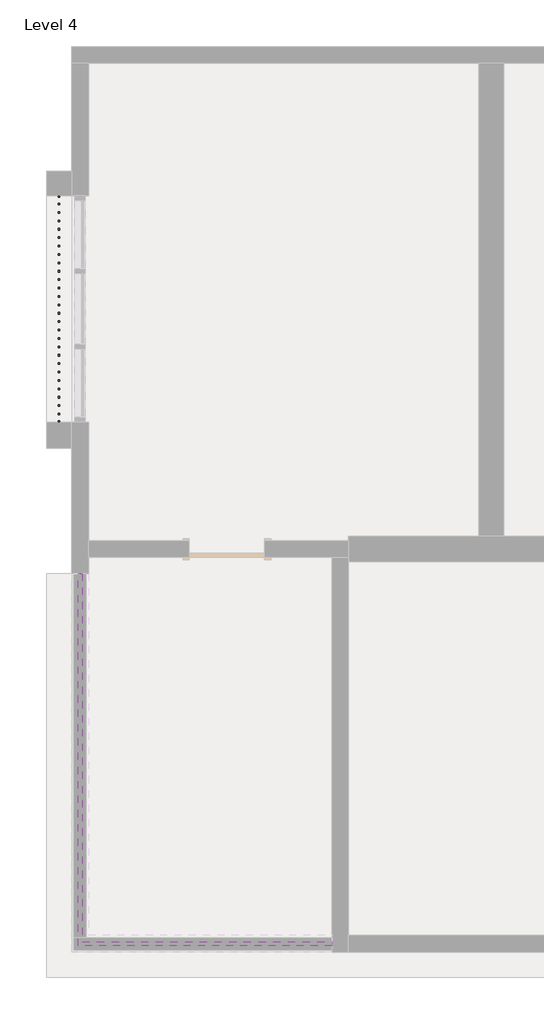
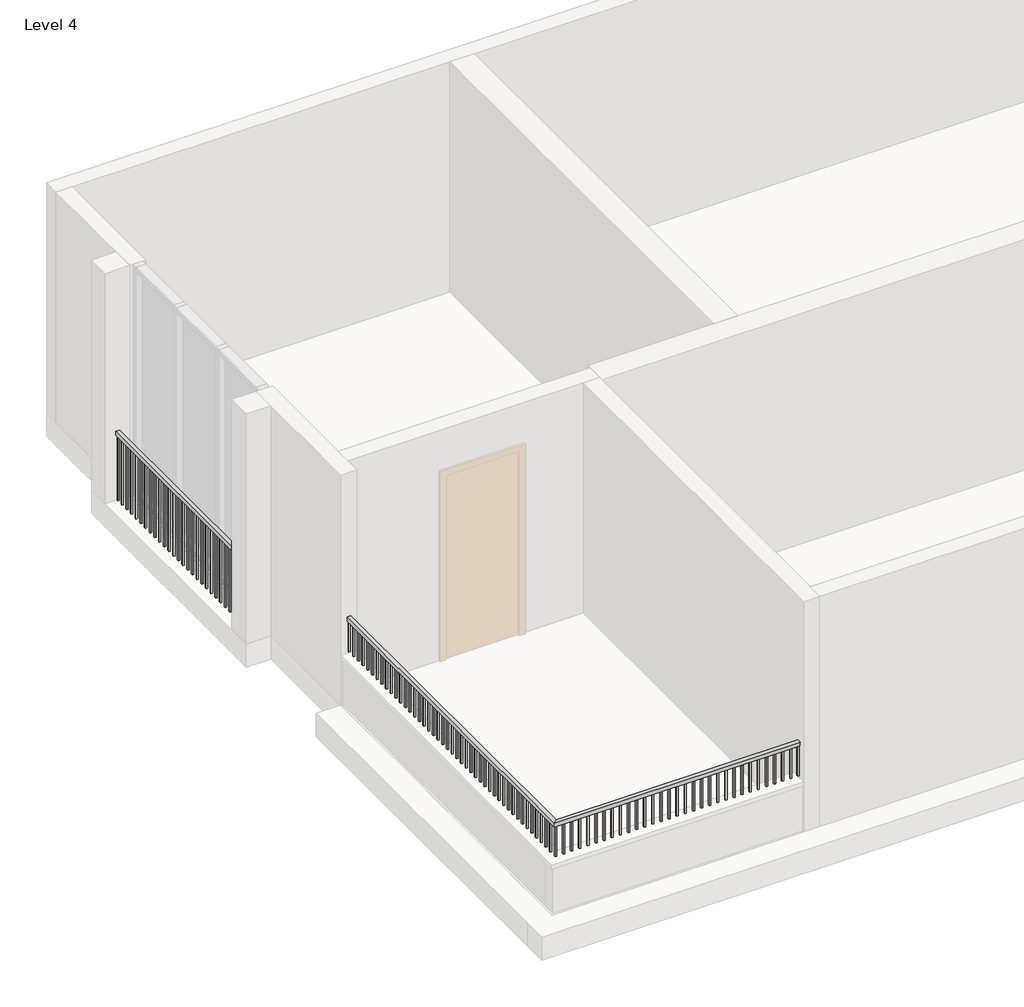
# One storey, part 2 of 2: 2 railings.
"""IFC4 building model written with IfcOpenShell, lengths in millimetres."""

from ifc_helpers import new_model, si_unit, frame, origin, place, context, project, spatial, polyline, outline, extrude, faceted_brep, element, save

model = new_model("IFC4")

# Units and contexts
model_context = context("Model", 3, world=origin())
ifc_project = project(units=[si_unit("LENGTHUNIT", "METRE", prefix="MILLI")], contexts=[model_context])

# Site, building, storey
site = spatial("IfcSite", under=ifc_project)
building = spatial("IfcBuilding", under=site)
storey = spatial("IfcBuildingStorey", under=building, Name="Level 4", Elevation=9144.0)

# Railings
placement = place(None, origin())
element("IfcRailing", 1, ObjectType="Handrail - Rectangular", at=placement, inside=storey, context=model_context, shape_type="SolidModel", body=[
    faceted_brep([(-15179.2169582, -9411.0617616, 11201.4), (-15179.2169582, -9411.0617616, 11150.6), (-15179.2169582, -9360.2617616, 11150.6), (-15179.2169582, -9360.2617616, 11201.4), (-18252.6169582, -9411.0617616, 11201.4), (-18252.6169582, -9411.0617616, 11150.6), (-18201.8169582, -9360.2617616, 11150.6), (-18201.8169582, -9360.2617616, 11201.4), (-18252.6169582, -4908.9117616, 11201.4), (-18201.8169582, -4908.9117616, 11201.4), (-18201.8169582, -4908.9117616, 11150.6), (-18252.6169582, -4908.9117616, 11150.6)], [[[0, 1, 2, 3]], [[1, 0, 4, 5]], [[2, 1, 5, 6]], [[3, 2, 6, 7]], [[0, 3, 7, 4]], [[8, 9, 10, 11]], [[5, 4, 8, 11]], [[6, 5, 11, 10]], [[7, 6, 10, 9]], [[4, 7, 9, 8]]]),
    extrude(outline(polyline([(-18217.6919582, -4924.7867616), (-18236.7419582, -4924.7867616), (-18236.7419582, -4905.7367616), (-18217.6919582, -4905.7367616), (-18217.6919582, -4924.7867616)])), frame((0.0, 0.0, 10744.2), z_axis=(0.0, 0.0, 1.0), x_axis=(1.0, 0.0, 0.0)), (0.0, 0.0, 1.0), 406.4),
    extrude(outline(polyline([(-18217.6919582, -5026.3867616), (-18236.7419582, -5026.3867616), (-18236.7419582, -5007.3367616), (-18217.6919582, -5007.3367616), (-18217.6919582, -5026.3867616)])), frame((0.0, 0.0, 10744.2), z_axis=(0.0, 0.0, 1.0), x_axis=(1.0, 0.0, 0.0)), (0.0, 0.0, 1.0), 406.4),
    extrude(outline(polyline([(-18217.6919582, -5127.9867616), (-18236.7419582, -5127.9867616), (-18236.7419582, -5108.9367616), (-18217.6919582, -5108.9367616), (-18217.6919582, -5127.9867616)])), frame((0.0, 0.0, 10744.2), z_axis=(0.0, 0.0, 1.0), x_axis=(1.0, 0.0, 0.0)), (0.0, 0.0, 1.0), 406.4),
    extrude(outline(polyline([(-18217.6919582, -5229.5867616), (-18236.7419582, -5229.5867616), (-18236.7419582, -5210.5367616), (-18217.6919582, -5210.5367616), (-18217.6919582, -5229.5867616)])), frame((0.0, 0.0, 10744.2), z_axis=(0.0, 0.0, 1.0), x_axis=(1.0, 0.0, 0.0)), (0.0, 0.0, 1.0), 406.4),
    extrude(outline(polyline([(-18217.6919582, -5331.1867616), (-18236.7419582, -5331.1867616), (-18236.7419582, -5312.1367616), (-18217.6919582, -5312.1367616), (-18217.6919582, -5331.1867616)])), frame((0.0, 0.0, 10744.2), z_axis=(0.0, 0.0, 1.0), x_axis=(1.0, 0.0, 0.0)), (0.0, 0.0, 1.0), 406.4),
    extrude(outline(polyline([(-18217.6919582, -5432.7867616), (-18236.7419582, -5432.7867616), (-18236.7419582, -5413.7367616), (-18217.6919582, -5413.7367616), (-18217.6919582, -5432.7867616)])), frame((0.0, 0.0, 10744.2), z_axis=(0.0, 0.0, 1.0), x_axis=(1.0, 0.0, 0.0)), (0.0, 0.0, 1.0), 406.4),
    extrude(outline(polyline([(-18217.6919582, -5534.3867616), (-18236.7419582, -5534.3867616), (-18236.7419582, -5515.3367616), (-18217.6919582, -5515.3367616), (-18217.6919582, -5534.3867616)])), frame((0.0, 0.0, 10744.2), z_axis=(0.0, 0.0, 1.0), x_axis=(1.0, 0.0, 0.0)), (0.0, 0.0, 1.0), 406.4),
    extrude(outline(polyline([(-18217.6919582, -5635.9867616), (-18236.7419582, -5635.9867616), (-18236.7419582, -5616.9367616), (-18217.6919582, -5616.9367616), (-18217.6919582, -5635.9867616)])), frame((0.0, 0.0, 10744.2), z_axis=(0.0, 0.0, 1.0), x_axis=(1.0, 0.0, 0.0)), (0.0, 0.0, 1.0), 406.4),
    extrude(outline(polyline([(-18217.6919582, -5737.5867616), (-18236.7419582, -5737.5867616), (-18236.7419582, -5718.5367616), (-18217.6919582, -5718.5367616), (-18217.6919582, -5737.5867616)])), frame((0.0, 0.0, 10744.2), z_axis=(0.0, 0.0, 1.0), x_axis=(1.0, 0.0, 0.0)), (0.0, 0.0, 1.0), 406.4),
    extrude(outline(polyline([(-18217.6919582, -5839.1867616), (-18236.7419582, -5839.1867616), (-18236.7419582, -5820.1367616), (-18217.6919582, -5820.1367616), (-18217.6919582, -5839.1867616)])), frame((0.0, 0.0, 10744.2), z_axis=(0.0, 0.0, 1.0), x_axis=(1.0, 0.0, 0.0)), (0.0, 0.0, 1.0), 406.4),
    extrude(outline(polyline([(-18217.6919582, -5940.7867616), (-18236.7419582, -5940.7867616), (-18236.7419582, -5921.7367616), (-18217.6919582, -5921.7367616), (-18217.6919582, -5940.7867616)])), frame((0.0, 0.0, 10744.2), z_axis=(0.0, 0.0, 1.0), x_axis=(1.0, 0.0, 0.0)), (0.0, 0.0, 1.0), 406.4),
    extrude(outline(polyline([(-18217.6919582, -6042.3867616), (-18236.7419582, -6042.3867616), (-18236.7419582, -6023.3367616), (-18217.6919582, -6023.3367616), (-18217.6919582, -6042.3867616)])), frame((0.0, 0.0, 10744.2), z_axis=(0.0, 0.0, 1.0), x_axis=(1.0, 0.0, 0.0)), (0.0, 0.0, 1.0), 406.4),
    extrude(outline(polyline([(-18217.6919582, -6143.9867616), (-18236.7419582, -6143.9867616), (-18236.7419582, -6124.9367616), (-18217.6919582, -6124.9367616), (-18217.6919582, -6143.9867616)])), frame((0.0, 0.0, 10744.2), z_axis=(0.0, 0.0, 1.0), x_axis=(1.0, 0.0, 0.0)), (0.0, 0.0, 1.0), 406.4),
    extrude(outline(polyline([(-18217.6919582, -6245.5867616), (-18236.7419582, -6245.5867616), (-18236.7419582, -6226.5367616), (-18217.6919582, -6226.5367616), (-18217.6919582, -6245.5867616)])), frame((0.0, 0.0, 10744.2), z_axis=(0.0, 0.0, 1.0), x_axis=(1.0, 0.0, 0.0)), (0.0, 0.0, 1.0), 406.4),
    extrude(outline(polyline([(-18217.6919582, -6347.1867616), (-18236.7419582, -6347.1867616), (-18236.7419582, -6328.1367616), (-18217.6919582, -6328.1367616), (-18217.6919582, -6347.1867616)])), frame((0.0, 0.0, 10744.2), z_axis=(0.0, 0.0, 1.0), x_axis=(1.0, 0.0, 0.0)), (0.0, 0.0, 1.0), 406.4),
    extrude(outline(polyline([(-18217.6919582, -6448.7867616), (-18236.7419582, -6448.7867616), (-18236.7419582, -6429.7367616), (-18217.6919582, -6429.7367616), (-18217.6919582, -6448.7867616)])), frame((0.0, 0.0, 10744.2), z_axis=(0.0, 0.0, 1.0), x_axis=(1.0, 0.0, 0.0)), (0.0, 0.0, 1.0), 406.4),
    extrude(outline(polyline([(-18217.6919582, -6550.3867616), (-18236.7419582, -6550.3867616), (-18236.7419582, -6531.3367616), (-18217.6919582, -6531.3367616), (-18217.6919582, -6550.3867616)])), frame((0.0, 0.0, 10744.2), z_axis=(0.0, 0.0, 1.0), x_axis=(1.0, 0.0, 0.0)), (0.0, 0.0, 1.0), 406.4),
    extrude(outline(polyline([(-18217.6919582, -6651.9867616), (-18236.7419582, -6651.9867616), (-18236.7419582, -6632.9367616), (-18217.6919582, -6632.9367616), (-18217.6919582, -6651.9867616)])), frame((0.0, 0.0, 10744.2), z_axis=(0.0, 0.0, 1.0), x_axis=(1.0, 0.0, 0.0)), (0.0, 0.0, 1.0), 406.4),
    extrude(outline(polyline([(-18217.6919582, -6753.5867616), (-18236.7419582, -6753.5867616), (-18236.7419582, -6734.5367616), (-18217.6919582, -6734.5367616), (-18217.6919582, -6753.5867616)])), frame((0.0, 0.0, 10744.2), z_axis=(0.0, 0.0, 1.0), x_axis=(1.0, 0.0, 0.0)), (0.0, 0.0, 1.0), 406.4),
    extrude(outline(polyline([(-18217.6919582, -6855.1867616), (-18236.7419582, -6855.1867616), (-18236.7419582, -6836.1367616), (-18217.6919582, -6836.1367616), (-18217.6919582, -6855.1867616)])), frame((0.0, 0.0, 10744.2), z_axis=(0.0, 0.0, 1.0), x_axis=(1.0, 0.0, 0.0)), (0.0, 0.0, 1.0), 406.4),
    extrude(outline(polyline([(-18217.6919582, -6956.7867616), (-18236.7419582, -6956.7867616), (-18236.7419582, -6937.7367616), (-18217.6919582, -6937.7367616), (-18217.6919582, -6956.7867616)])), frame((0.0, 0.0, 10744.2), z_axis=(0.0, 0.0, 1.0), x_axis=(1.0, 0.0, 0.0)), (0.0, 0.0, 1.0), 406.4),
    extrude(outline(polyline([(-18217.6919582, -7058.3867616), (-18236.7419582, -7058.3867616), (-18236.7419582, -7039.3367616), (-18217.6919582, -7039.3367616), (-18217.6919582, -7058.3867616)])), frame((0.0, 0.0, 10744.2), z_axis=(0.0, 0.0, 1.0), x_axis=(1.0, 0.0, 0.0)), (0.0, 0.0, 1.0), 406.4),
    extrude(outline(polyline([(-18217.6919582, -7159.9867616), (-18236.7419582, -7159.9867616), (-18236.7419582, -7140.9367616), (-18217.6919582, -7140.9367616), (-18217.6919582, -7159.9867616)])), frame((0.0, 0.0, 10744.2), z_axis=(0.0, 0.0, 1.0), x_axis=(1.0, 0.0, 0.0)), (0.0, 0.0, 1.0), 406.4),
    extrude(outline(polyline([(-18217.6919582, -7261.5867616), (-18236.7419582, -7261.5867616), (-18236.7419582, -7242.5367616), (-18217.6919582, -7242.5367616), (-18217.6919582, -7261.5867616)])), frame((0.0, 0.0, 10744.2), z_axis=(0.0, 0.0, 1.0), x_axis=(1.0, 0.0, 0.0)), (0.0, 0.0, 1.0), 406.4),
    extrude(outline(polyline([(-18217.6919582, -7363.1867616), (-18236.7419582, -7363.1867616), (-18236.7419582, -7344.1367616), (-18217.6919582, -7344.1367616), (-18217.6919582, -7363.1867616)])), frame((0.0, 0.0, 10744.2), z_axis=(0.0, 0.0, 1.0), x_axis=(1.0, 0.0, 0.0)), (0.0, 0.0, 1.0), 406.4),
    extrude(outline(polyline([(-18217.6919582, -7464.7867616), (-18236.7419582, -7464.7867616), (-18236.7419582, -7445.7367616), (-18217.6919582, -7445.7367616), (-18217.6919582, -7464.7867616)])), frame((0.0, 0.0, 10744.2), z_axis=(0.0, 0.0, 1.0), x_axis=(1.0, 0.0, 0.0)), (0.0, 0.0, 1.0), 406.4),
    extrude(outline(polyline([(-18217.6919582, -7566.3867616), (-18236.7419582, -7566.3867616), (-18236.7419582, -7547.3367616), (-18217.6919582, -7547.3367616), (-18217.6919582, -7566.3867616)])), frame((0.0, 0.0, 10744.2), z_axis=(0.0, 0.0, 1.0), x_axis=(1.0, 0.0, 0.0)), (0.0, 0.0, 1.0), 406.4),
    extrude(outline(polyline([(-18217.6919582, -7667.9867616), (-18236.7419582, -7667.9867616), (-18236.7419582, -7648.9367616), (-18217.6919582, -7648.9367616), (-18217.6919582, -7667.9867616)])), frame((0.0, 0.0, 10744.2), z_axis=(0.0, 0.0, 1.0), x_axis=(1.0, 0.0, 0.0)), (0.0, 0.0, 1.0), 406.4),
    extrude(outline(polyline([(-18217.6919582, -7769.5867616), (-18236.7419582, -7769.5867616), (-18236.7419582, -7750.5367616), (-18217.6919582, -7750.5367616), (-18217.6919582, -7769.5867616)])), frame((0.0, 0.0, 10744.2), z_axis=(0.0, 0.0, 1.0), x_axis=(1.0, 0.0, 0.0)), (0.0, 0.0, 1.0), 406.4),
    extrude(outline(polyline([(-18217.6919582, -7871.1867616), (-18236.7419582, -7871.1867616), (-18236.7419582, -7852.1367616), (-18217.6919582, -7852.1367616), (-18217.6919582, -7871.1867616)])), frame((0.0, 0.0, 10744.2), z_axis=(0.0, 0.0, 1.0), x_axis=(1.0, 0.0, 0.0)), (0.0, 0.0, 1.0), 406.4),
    extrude(outline(polyline([(-18217.6919582, -7972.7867616), (-18236.7419582, -7972.7867616), (-18236.7419582, -7953.7367616), (-18217.6919582, -7953.7367616), (-18217.6919582, -7972.7867616)])), frame((0.0, 0.0, 10744.2), z_axis=(0.0, 0.0, 1.0), x_axis=(1.0, 0.0, 0.0)), (0.0, 0.0, 1.0), 406.4),
    extrude(outline(polyline([(-18217.6919582, -8074.3867616), (-18236.7419582, -8074.3867616), (-18236.7419582, -8055.3367616), (-18217.6919582, -8055.3367616), (-18217.6919582, -8074.3867616)])), frame((0.0, 0.0, 10744.2), z_axis=(0.0, 0.0, 1.0), x_axis=(1.0, 0.0, 0.0)), (0.0, 0.0, 1.0), 406.4),
    extrude(outline(polyline([(-18217.6919582, -8175.9867616), (-18236.7419582, -8175.9867616), (-18236.7419582, -8156.9367616), (-18217.6919582, -8156.9367616), (-18217.6919582, -8175.9867616)])), frame((0.0, 0.0, 10744.2), z_axis=(0.0, 0.0, 1.0), x_axis=(1.0, 0.0, 0.0)), (0.0, 0.0, 1.0), 406.4),
    extrude(outline(polyline([(-18217.6919582, -8277.5867616), (-18236.7419582, -8277.5867616), (-18236.7419582, -8258.5367616), (-18217.6919582, -8258.5367616), (-18217.6919582, -8277.5867616)])), frame((0.0, 0.0, 10744.2), z_axis=(0.0, 0.0, 1.0), x_axis=(1.0, 0.0, 0.0)), (0.0, 0.0, 1.0), 406.4),
    extrude(outline(polyline([(-18217.6919582, -8379.1867616), (-18236.7419582, -8379.1867616), (-18236.7419582, -8360.1367616), (-18217.6919582, -8360.1367616), (-18217.6919582, -8379.1867616)])), frame((0.0, 0.0, 10744.2), z_axis=(0.0, 0.0, 1.0), x_axis=(1.0, 0.0, 0.0)), (0.0, 0.0, 1.0), 406.4),
    extrude(outline(polyline([(-18217.6919582, -8480.7867616), (-18236.7419582, -8480.7867616), (-18236.7419582, -8461.7367616), (-18217.6919582, -8461.7367616), (-18217.6919582, -8480.7867616)])), frame((0.0, 0.0, 10744.2), z_axis=(0.0, 0.0, 1.0), x_axis=(1.0, 0.0, 0.0)), (0.0, 0.0, 1.0), 406.4),
    extrude(outline(polyline([(-18217.6919582, -8582.3867616), (-18236.7419582, -8582.3867616), (-18236.7419582, -8563.3367616), (-18217.6919582, -8563.3367616), (-18217.6919582, -8582.3867616)])), frame((0.0, 0.0, 10744.2), z_axis=(0.0, 0.0, 1.0), x_axis=(1.0, 0.0, 0.0)), (0.0, 0.0, 1.0), 406.4),
    extrude(outline(polyline([(-18217.6919582, -8683.9867616), (-18236.7419582, -8683.9867616), (-18236.7419582, -8664.9367616), (-18217.6919582, -8664.9367616), (-18217.6919582, -8683.9867616)])), frame((0.0, 0.0, 10744.2), z_axis=(0.0, 0.0, 1.0), x_axis=(1.0, 0.0, 0.0)), (0.0, 0.0, 1.0), 406.4),
    extrude(outline(polyline([(-18217.6919582, -8785.5867616), (-18236.7419582, -8785.5867616), (-18236.7419582, -8766.5367616), (-18217.6919582, -8766.5367616), (-18217.6919582, -8785.5867616)])), frame((0.0, 0.0, 10744.2), z_axis=(0.0, 0.0, 1.0), x_axis=(1.0, 0.0, 0.0)), (0.0, 0.0, 1.0), 406.4),
    extrude(outline(polyline([(-18217.6919582, -8887.1867616), (-18236.7419582, -8887.1867616), (-18236.7419582, -8868.1367616), (-18217.6919582, -8868.1367616), (-18217.6919582, -8887.1867616)])), frame((0.0, 0.0, 10744.2), z_axis=(0.0, 0.0, 1.0), x_axis=(1.0, 0.0, 0.0)), (0.0, 0.0, 1.0), 406.4),
    extrude(outline(polyline([(-18217.6919582, -8988.7867616), (-18236.7419582, -8988.7867616), (-18236.7419582, -8969.7367616), (-18217.6919582, -8969.7367616), (-18217.6919582, -8988.7867616)])), frame((0.0, 0.0, 10744.2), z_axis=(0.0, 0.0, 1.0), x_axis=(1.0, 0.0, 0.0)), (0.0, 0.0, 1.0), 406.4),
    extrude(outline(polyline([(-18217.6919582, -9090.3867616), (-18236.7419582, -9090.3867616), (-18236.7419582, -9071.3367616), (-18217.6919582, -9071.3367616), (-18217.6919582, -9090.3867616)])), frame((0.0, 0.0, 10744.2), z_axis=(0.0, 0.0, 1.0), x_axis=(1.0, 0.0, 0.0)), (0.0, 0.0, 1.0), 406.4),
    extrude(outline(polyline([(-18217.6919582, -9191.9867616), (-18236.7419582, -9191.9867616), (-18236.7419582, -9172.9367616), (-18217.6919582, -9172.9367616), (-18217.6919582, -9191.9867616)])), frame((0.0, 0.0, 10744.2), z_axis=(0.0, 0.0, 1.0), x_axis=(1.0, 0.0, 0.0)), (0.0, 0.0, 1.0), 406.4),
    extrude(outline(polyline([(-18217.6919582, -9293.5867616), (-18236.7419582, -9293.5867616), (-18236.7419582, -9274.5367616), (-18217.6919582, -9274.5367616), (-18217.6919582, -9293.5867616)])), frame((0.0, 0.0, 10744.2), z_axis=(0.0, 0.0, 1.0), x_axis=(1.0, 0.0, 0.0)), (0.0, 0.0, 1.0), 406.4),
    extrude(outline(polyline([(-18116.0919582, -9376.1367616), (-18116.0919582, -9395.1867616), (-18135.1419582, -9395.1867616), (-18135.1419582, -9376.1367616), (-18116.0919582, -9376.1367616)])), frame((0.0, 0.0, 10744.2), z_axis=(0.0, 0.0, 1.0), x_axis=(1.0, 0.0, 0.0)), (0.0, 0.0, 1.0), 406.4),
    extrude(outline(polyline([(-18014.4919582, -9376.1367616), (-18014.4919582, -9395.1867616), (-18033.5419582, -9395.1867616), (-18033.5419582, -9376.1367616), (-18014.4919582, -9376.1367616)])), frame((0.0, 0.0, 10744.2), z_axis=(0.0, 0.0, 1.0), x_axis=(1.0, 0.0, 0.0)), (0.0, 0.0, 1.0), 406.4),
    extrude(outline(polyline([(-17912.8919582, -9376.1367616), (-17912.8919582, -9395.1867616), (-17931.9419582, -9395.1867616), (-17931.9419582, -9376.1367616), (-17912.8919582, -9376.1367616)])), frame((0.0, 0.0, 10744.2), z_axis=(0.0, 0.0, 1.0), x_axis=(1.0, 0.0, 0.0)), (0.0, 0.0, 1.0), 406.4),
    extrude(outline(polyline([(-17811.2919582, -9376.1367616), (-17811.2919582, -9395.1867616), (-17830.3419582, -9395.1867616), (-17830.3419582, -9376.1367616), (-17811.2919582, -9376.1367616)])), frame((0.0, 0.0, 10744.2), z_axis=(0.0, 0.0, 1.0), x_axis=(1.0, 0.0, 0.0)), (0.0, 0.0, 1.0), 406.4),
    extrude(outline(polyline([(-17709.6919582, -9376.1367616), (-17709.6919582, -9395.1867616), (-17728.7419582, -9395.1867616), (-17728.7419582, -9376.1367616), (-17709.6919582, -9376.1367616)])), frame((0.0, 0.0, 10744.2), z_axis=(0.0, 0.0, 1.0), x_axis=(1.0, 0.0, 0.0)), (0.0, 0.0, 1.0), 406.4),
    extrude(outline(polyline([(-17608.0919582, -9376.1367616), (-17608.0919582, -9395.1867616), (-17627.1419582, -9395.1867616), (-17627.1419582, -9376.1367616), (-17608.0919582, -9376.1367616)])), frame((0.0, 0.0, 10744.2), z_axis=(0.0, 0.0, 1.0), x_axis=(1.0, 0.0, 0.0)), (0.0, 0.0, 1.0), 406.4),
    extrude(outline(polyline([(-17506.4919582, -9376.1367616), (-17506.4919582, -9395.1867616), (-17525.5419582, -9395.1867616), (-17525.5419582, -9376.1367616), (-17506.4919582, -9376.1367616)])), frame((0.0, 0.0, 10744.2), z_axis=(0.0, 0.0, 1.0), x_axis=(1.0, 0.0, 0.0)), (0.0, 0.0, 1.0), 406.4),
    extrude(outline(polyline([(-17404.8919582, -9376.1367616), (-17404.8919582, -9395.1867616), (-17423.9419582, -9395.1867616), (-17423.9419582, -9376.1367616), (-17404.8919582, -9376.1367616)])), frame((0.0, 0.0, 10744.2), z_axis=(0.0, 0.0, 1.0), x_axis=(1.0, 0.0, 0.0)), (0.0, 0.0, 1.0), 406.4),
    extrude(outline(polyline([(-17303.2919582, -9376.1367616), (-17303.2919582, -9395.1867616), (-17322.3419582, -9395.1867616), (-17322.3419582, -9376.1367616), (-17303.2919582, -9376.1367616)])), frame((0.0, 0.0, 10744.2), z_axis=(0.0, 0.0, 1.0), x_axis=(1.0, 0.0, 0.0)), (0.0, 0.0, 1.0), 406.4),
    extrude(outline(polyline([(-17201.6919582, -9376.1367616), (-17201.6919582, -9395.1867616), (-17220.7419582, -9395.1867616), (-17220.7419582, -9376.1367616), (-17201.6919582, -9376.1367616)])), frame((0.0, 0.0, 10744.2), z_axis=(0.0, 0.0, 1.0), x_axis=(1.0, 0.0, 0.0)), (0.0, 0.0, 1.0), 406.4),
    extrude(outline(polyline([(-17100.0919582, -9376.1367616), (-17100.0919582, -9395.1867616), (-17119.1419582, -9395.1867616), (-17119.1419582, -9376.1367616), (-17100.0919582, -9376.1367616)])), frame((0.0, 0.0, 10744.2), z_axis=(0.0, 0.0, 1.0), x_axis=(1.0, 0.0, 0.0)), (0.0, 0.0, 1.0), 406.4),
    extrude(outline(polyline([(-16998.4919582, -9376.1367616), (-16998.4919582, -9395.1867616), (-17017.5419582, -9395.1867616), (-17017.5419582, -9376.1367616), (-16998.4919582, -9376.1367616)])), frame((0.0, 0.0, 10744.2), z_axis=(0.0, 0.0, 1.0), x_axis=(1.0, 0.0, 0.0)), (0.0, 0.0, 1.0), 406.4),
    extrude(outline(polyline([(-16896.8919582, -9376.1367616), (-16896.8919582, -9395.1867616), (-16915.9419582, -9395.1867616), (-16915.9419582, -9376.1367616), (-16896.8919582, -9376.1367616)])), frame((0.0, 0.0, 10744.2), z_axis=(0.0, 0.0, 1.0), x_axis=(1.0, 0.0, 0.0)), (0.0, 0.0, 1.0), 406.4),
    extrude(outline(polyline([(-16795.2919582, -9376.1367616), (-16795.2919582, -9395.1867616), (-16814.3419582, -9395.1867616), (-16814.3419582, -9376.1367616), (-16795.2919582, -9376.1367616)])), frame((0.0, 0.0, 10744.2), z_axis=(0.0, 0.0, 1.0), x_axis=(1.0, 0.0, 0.0)), (0.0, 0.0, 1.0), 406.4),
    extrude(outline(polyline([(-16693.6919582, -9376.1367616), (-16693.6919582, -9395.1867616), (-16712.7419582, -9395.1867616), (-16712.7419582, -9376.1367616), (-16693.6919582, -9376.1367616)])), frame((0.0, 0.0, 10744.2), z_axis=(0.0, 0.0, 1.0), x_axis=(1.0, 0.0, 0.0)), (0.0, 0.0, 1.0), 406.4),
    extrude(outline(polyline([(-16592.0919582, -9376.1367616), (-16592.0919582, -9395.1867616), (-16611.1419582, -9395.1867616), (-16611.1419582, -9376.1367616), (-16592.0919582, -9376.1367616)])), frame((0.0, 0.0, 10744.2), z_axis=(0.0, 0.0, 1.0), x_axis=(1.0, 0.0, 0.0)), (0.0, 0.0, 1.0), 406.4),
    extrude(outline(polyline([(-16490.4919582, -9376.1367616), (-16490.4919582, -9395.1867616), (-16509.5419582, -9395.1867616), (-16509.5419582, -9376.1367616), (-16490.4919582, -9376.1367616)])), frame((0.0, 0.0, 10744.2), z_axis=(0.0, 0.0, 1.0), x_axis=(1.0, 0.0, 0.0)), (0.0, 0.0, 1.0), 406.4),
    extrude(outline(polyline([(-16388.8919582, -9376.1367616), (-16388.8919582, -9395.1867616), (-16407.9419582, -9395.1867616), (-16407.9419582, -9376.1367616), (-16388.8919582, -9376.1367616)])), frame((0.0, 0.0, 10744.2), z_axis=(0.0, 0.0, 1.0), x_axis=(1.0, 0.0, 0.0)), (0.0, 0.0, 1.0), 406.4),
    extrude(outline(polyline([(-16287.2919582, -9376.1367616), (-16287.2919582, -9395.1867616), (-16306.3419582, -9395.1867616), (-16306.3419582, -9376.1367616), (-16287.2919582, -9376.1367616)])), frame((0.0, 0.0, 10744.2), z_axis=(0.0, 0.0, 1.0), x_axis=(1.0, 0.0, 0.0)), (0.0, 0.0, 1.0), 406.4),
    extrude(outline(polyline([(-16185.6919582, -9376.1367616), (-16185.6919582, -9395.1867616), (-16204.7419582, -9395.1867616), (-16204.7419582, -9376.1367616), (-16185.6919582, -9376.1367616)])), frame((0.0, 0.0, 10744.2), z_axis=(0.0, 0.0, 1.0), x_axis=(1.0, 0.0, 0.0)), (0.0, 0.0, 1.0), 406.4),
    extrude(outline(polyline([(-16084.0919582, -9376.1367616), (-16084.0919582, -9395.1867616), (-16103.1419582, -9395.1867616), (-16103.1419582, -9376.1367616), (-16084.0919582, -9376.1367616)])), frame((0.0, 0.0, 10744.2), z_axis=(0.0, 0.0, 1.0), x_axis=(1.0, 0.0, 0.0)), (0.0, 0.0, 1.0), 406.4),
    extrude(outline(polyline([(-15982.4919582, -9376.1367616), (-15982.4919582, -9395.1867616), (-16001.5419582, -9395.1867616), (-16001.5419582, -9376.1367616), (-15982.4919582, -9376.1367616)])), frame((0.0, 0.0, 10744.2), z_axis=(0.0, 0.0, 1.0), x_axis=(1.0, 0.0, 0.0)), (0.0, 0.0, 1.0), 406.4),
    extrude(outline(polyline([(-15880.8919582, -9376.1367616), (-15880.8919582, -9395.1867616), (-15899.9419582, -9395.1867616), (-15899.9419582, -9376.1367616), (-15880.8919582, -9376.1367616)])), frame((0.0, 0.0, 10744.2), z_axis=(0.0, 0.0, 1.0), x_axis=(1.0, 0.0, 0.0)), (0.0, 0.0, 1.0), 406.4),
    extrude(outline(polyline([(-15779.2919582, -9376.1367616), (-15779.2919582, -9395.1867616), (-15798.3419582, -9395.1867616), (-15798.3419582, -9376.1367616), (-15779.2919582, -9376.1367616)])), frame((0.0, 0.0, 10744.2), z_axis=(0.0, 0.0, 1.0), x_axis=(1.0, 0.0, 0.0)), (0.0, 0.0, 1.0), 406.4),
    extrude(outline(polyline([(-15677.6919582, -9376.1367616), (-15677.6919582, -9395.1867616), (-15696.7419582, -9395.1867616), (-15696.7419582, -9376.1367616), (-15677.6919582, -9376.1367616)])), frame((0.0, 0.0, 10744.2), z_axis=(0.0, 0.0, 1.0), x_axis=(1.0, 0.0, 0.0)), (0.0, 0.0, 1.0), 406.4),
    extrude(outline(polyline([(-15576.0919582, -9376.1367616), (-15576.0919582, -9395.1867616), (-15595.1419582, -9395.1867616), (-15595.1419582, -9376.1367616), (-15576.0919582, -9376.1367616)])), frame((0.0, 0.0, 10744.2), z_axis=(0.0, 0.0, 1.0), x_axis=(1.0, 0.0, 0.0)), (0.0, 0.0, 1.0), 406.4),
    extrude(outline(polyline([(-15474.4919582, -9376.1367616), (-15474.4919582, -9395.1867616), (-15493.5419582, -9395.1867616), (-15493.5419582, -9376.1367616), (-15474.4919582, -9376.1367616)])), frame((0.0, 0.0, 10744.2), z_axis=(0.0, 0.0, 1.0), x_axis=(1.0, 0.0, 0.0)), (0.0, 0.0, 1.0), 406.4),
    extrude(outline(polyline([(-15372.8919582, -9376.1367616), (-15372.8919582, -9395.1867616), (-15391.9419582, -9395.1867616), (-15391.9419582, -9376.1367616), (-15372.8919582, -9376.1367616)])), frame((0.0, 0.0, 10744.2), z_axis=(0.0, 0.0, 1.0), x_axis=(1.0, 0.0, 0.0)), (0.0, 0.0, 1.0), 406.4),
    extrude(outline(polyline([(-15271.2919582, -9376.1367616), (-15271.2919582, -9395.1867616), (-15290.3419582, -9395.1867616), (-15290.3419582, -9376.1367616), (-15271.2919582, -9376.1367616)])), frame((0.0, 0.0, 10744.2), z_axis=(0.0, 0.0, 1.0), x_axis=(1.0, 0.0, 0.0)), (0.0, 0.0, 1.0), 406.4),
    extrude(outline(polyline([(-18217.6919582, -9376.1367616), (-18217.6919582, -9395.1867616), (-18236.7419582, -9395.1867616), (-18236.7419582, -9376.1367616), (-18217.6919582, -9376.1367616)])), frame((0.0, 0.0, 10744.2), z_axis=(0.0, 0.0, 1.0), x_axis=(1.0, 0.0, 0.0)), (0.0, 0.0, 1.0), 406.4),
    extrude(outline(polyline([(-18217.6919582, -4927.9617616), (-18236.7419582, -4927.9617616), (-18236.7419582, -4908.9117616), (-18217.6919582, -4908.9117616), (-18217.6919582, -4927.9617616)])), frame((0.0, 0.0, 10744.2), z_axis=(0.0, 0.0, 1.0), x_axis=(1.0, 0.0, 0.0)), (0.0, 0.0, 1.0), 406.4),
    extrude(outline(polyline([(-15179.2169582, -9376.1367616), (-15179.2169582, -9395.1867616), (-15198.2669582, -9395.1867616), (-15198.2669582, -9376.1367616), (-15179.2169582, -9376.1367616)])), frame((0.0, 0.0, 10744.2), z_axis=(0.0, 0.0, 1.0), x_axis=(1.0, 0.0, 0.0)), (0.0, 0.0, 1.0), 406.4),
])
element("IfcRailing", 2, ObjectType="Handrail - Rectangular 2", at=placement, inside=storey, context=model_context, shape_type="SweptSolid", body=[
    extrude(outline(polyline([(-18506.6169582, -336.9117616), (-18455.8169582, -336.9117616), (-18455.8169582, -3080.1117616), (-18506.6169582, -3080.1117616), (-18506.6169582, -336.9117616)])), frame((0.0, 0.0, 10922.0), z_axis=(0.0, 0.0, 1.0), x_axis=(1.0, 0.0, 0.0)), (0.0, 0.0, 1.0), 50.8),
    extrude(outline(polyline([(-18490.7419582, -2968.9867616), (-18471.6919582, -2968.9867616), (-18471.6919582, -2988.0367616), (-18490.7419582, -2988.0367616), (-18490.7419582, -2968.9867616)])), frame((0.0, 0.0, 10058.4), z_axis=(0.0, 0.0, 1.0), x_axis=(1.0, 0.0, 0.0)), (0.0, 0.0, 1.0), 863.6),
    extrude(outline(polyline([(-18490.7419582, -2867.3867616), (-18471.6919582, -2867.3867616), (-18471.6919582, -2886.4367616), (-18490.7419582, -2886.4367616), (-18490.7419582, -2867.3867616)])), frame((0.0, 0.0, 10058.4), z_axis=(0.0, 0.0, 1.0), x_axis=(1.0, 0.0, 0.0)), (0.0, 0.0, 1.0), 863.6),
    extrude(outline(polyline([(-18490.7419582, -2765.7867616), (-18471.6919582, -2765.7867616), (-18471.6919582, -2784.8367616), (-18490.7419582, -2784.8367616), (-18490.7419582, -2765.7867616)])), frame((0.0, 0.0, 10058.4), z_axis=(0.0, 0.0, 1.0), x_axis=(1.0, 0.0, 0.0)), (0.0, 0.0, 1.0), 863.6),
    extrude(outline(polyline([(-18490.7419582, -2664.1867616), (-18471.6919582, -2664.1867616), (-18471.6919582, -2683.2367616), (-18490.7419582, -2683.2367616), (-18490.7419582, -2664.1867616)])), frame((0.0, 0.0, 10058.4), z_axis=(0.0, 0.0, 1.0), x_axis=(1.0, 0.0, 0.0)), (0.0, 0.0, 1.0), 863.6),
    extrude(outline(polyline([(-18490.7419582, -2562.5867616), (-18471.6919582, -2562.5867616), (-18471.6919582, -2581.6367616), (-18490.7419582, -2581.6367616), (-18490.7419582, -2562.5867616)])), frame((0.0, 0.0, 10058.4), z_axis=(0.0, 0.0, 1.0), x_axis=(1.0, 0.0, 0.0)), (0.0, 0.0, 1.0), 863.6),
    extrude(outline(polyline([(-18490.7419582, -2460.9867616), (-18471.6919582, -2460.9867616), (-18471.6919582, -2480.0367616), (-18490.7419582, -2480.0367616), (-18490.7419582, -2460.9867616)])), frame((0.0, 0.0, 10058.4), z_axis=(0.0, 0.0, 1.0), x_axis=(1.0, 0.0, 0.0)), (0.0, 0.0, 1.0), 863.6),
    extrude(outline(polyline([(-18490.7419582, -2359.3867616), (-18471.6919582, -2359.3867616), (-18471.6919582, -2378.4367616), (-18490.7419582, -2378.4367616), (-18490.7419582, -2359.3867616)])), frame((0.0, 0.0, 10058.4), z_axis=(0.0, 0.0, 1.0), x_axis=(1.0, 0.0, 0.0)), (0.0, 0.0, 1.0), 863.6),
    extrude(outline(polyline([(-18490.7419582, -2257.7867616), (-18471.6919582, -2257.7867616), (-18471.6919582, -2276.8367616), (-18490.7419582, -2276.8367616), (-18490.7419582, -2257.7867616)])), frame((0.0, 0.0, 10058.4), z_axis=(0.0, 0.0, 1.0), x_axis=(1.0, 0.0, 0.0)), (0.0, 0.0, 1.0), 863.6),
    extrude(outline(polyline([(-18490.7419582, -2156.1867616), (-18471.6919582, -2156.1867616), (-18471.6919582, -2175.2367616), (-18490.7419582, -2175.2367616), (-18490.7419582, -2156.1867616)])), frame((0.0, 0.0, 10058.4), z_axis=(0.0, 0.0, 1.0), x_axis=(1.0, 0.0, 0.0)), (0.0, 0.0, 1.0), 863.6),
    extrude(outline(polyline([(-18490.7419582, -2054.5867616), (-18471.6919582, -2054.5867616), (-18471.6919582, -2073.6367616), (-18490.7419582, -2073.6367616), (-18490.7419582, -2054.5867616)])), frame((0.0, 0.0, 10058.4), z_axis=(0.0, 0.0, 1.0), x_axis=(1.0, 0.0, 0.0)), (0.0, 0.0, 1.0), 863.6),
    extrude(outline(polyline([(-18490.7419582, -1952.9867616), (-18471.6919582, -1952.9867616), (-18471.6919582, -1972.0367616), (-18490.7419582, -1972.0367616), (-18490.7419582, -1952.9867616)])), frame((0.0, 0.0, 10058.4), z_axis=(0.0, 0.0, 1.0), x_axis=(1.0, 0.0, 0.0)), (0.0, 0.0, 1.0), 863.6),
    extrude(outline(polyline([(-18490.7419582, -1851.3867616), (-18471.6919582, -1851.3867616), (-18471.6919582, -1870.4367616), (-18490.7419582, -1870.4367616), (-18490.7419582, -1851.3867616)])), frame((0.0, 0.0, 10058.4), z_axis=(0.0, 0.0, 1.0), x_axis=(1.0, 0.0, 0.0)), (0.0, 0.0, 1.0), 863.6),
    extrude(outline(polyline([(-18490.7419582, -1749.7867616), (-18471.6919582, -1749.7867616), (-18471.6919582, -1768.8367616), (-18490.7419582, -1768.8367616), (-18490.7419582, -1749.7867616)])), frame((0.0, 0.0, 10058.4), z_axis=(0.0, 0.0, 1.0), x_axis=(1.0, 0.0, 0.0)), (0.0, 0.0, 1.0), 863.6),
    extrude(outline(polyline([(-18490.7419582, -1648.1867616), (-18471.6919582, -1648.1867616), (-18471.6919582, -1667.2367616), (-18490.7419582, -1667.2367616), (-18490.7419582, -1648.1867616)])), frame((0.0, 0.0, 10058.4), z_axis=(0.0, 0.0, 1.0), x_axis=(1.0, 0.0, 0.0)), (0.0, 0.0, 1.0), 863.6),
    extrude(outline(polyline([(-18490.7419582, -1546.5867616), (-18471.6919582, -1546.5867616), (-18471.6919582, -1565.6367616), (-18490.7419582, -1565.6367616), (-18490.7419582, -1546.5867616)])), frame((0.0, 0.0, 10058.4), z_axis=(0.0, 0.0, 1.0), x_axis=(1.0, 0.0, 0.0)), (0.0, 0.0, 1.0), 863.6),
    extrude(outline(polyline([(-18490.7419582, -1444.9867616), (-18471.6919582, -1444.9867616), (-18471.6919582, -1464.0367616), (-18490.7419582, -1464.0367616), (-18490.7419582, -1444.9867616)])), frame((0.0, 0.0, 10058.4), z_axis=(0.0, 0.0, 1.0), x_axis=(1.0, 0.0, 0.0)), (0.0, 0.0, 1.0), 863.6),
    extrude(outline(polyline([(-18490.7419582, -1343.3867616), (-18471.6919582, -1343.3867616), (-18471.6919582, -1362.4367616), (-18490.7419582, -1362.4367616), (-18490.7419582, -1343.3867616)])), frame((0.0, 0.0, 10058.4), z_axis=(0.0, 0.0, 1.0), x_axis=(1.0, 0.0, 0.0)), (0.0, 0.0, 1.0), 863.6),
    extrude(outline(polyline([(-18490.7419582, -1241.7867616), (-18471.6919582, -1241.7867616), (-18471.6919582, -1260.8367616), (-18490.7419582, -1260.8367616), (-18490.7419582, -1241.7867616)])), frame((0.0, 0.0, 10058.4), z_axis=(0.0, 0.0, 1.0), x_axis=(1.0, 0.0, 0.0)), (0.0, 0.0, 1.0), 863.6),
    extrude(outline(polyline([(-18490.7419582, -1140.1867616), (-18471.6919582, -1140.1867616), (-18471.6919582, -1159.2367616), (-18490.7419582, -1159.2367616), (-18490.7419582, -1140.1867616)])), frame((0.0, 0.0, 10058.4), z_axis=(0.0, 0.0, 1.0), x_axis=(1.0, 0.0, 0.0)), (0.0, 0.0, 1.0), 863.6),
    extrude(outline(polyline([(-18490.7419582, -1038.5867616), (-18471.6919582, -1038.5867616), (-18471.6919582, -1057.6367616), (-18490.7419582, -1057.6367616), (-18490.7419582, -1038.5867616)])), frame((0.0, 0.0, 10058.4), z_axis=(0.0, 0.0, 1.0), x_axis=(1.0, 0.0, 0.0)), (0.0, 0.0, 1.0), 863.6),
    extrude(outline(polyline([(-18490.7419582, -936.9867616), (-18471.6919582, -936.9867616), (-18471.6919582, -956.0367616), (-18490.7419582, -956.0367616), (-18490.7419582, -936.9867616)])), frame((0.0, 0.0, 10058.4), z_axis=(0.0, 0.0, 1.0), x_axis=(1.0, 0.0, 0.0)), (0.0, 0.0, 1.0), 863.6),
    extrude(outline(polyline([(-18490.7419582, -835.3867616), (-18471.6919582, -835.3867616), (-18471.6919582, -854.4367616), (-18490.7419582, -854.4367616), (-18490.7419582, -835.3867616)])), frame((0.0, 0.0, 10058.4), z_axis=(0.0, 0.0, 1.0), x_axis=(1.0, 0.0, 0.0)), (0.0, 0.0, 1.0), 863.6),
    extrude(outline(polyline([(-18490.7419582, -733.7867616), (-18471.6919582, -733.7867616), (-18471.6919582, -752.8367616), (-18490.7419582, -752.8367616), (-18490.7419582, -733.7867616)])), frame((0.0, 0.0, 10058.4), z_axis=(0.0, 0.0, 1.0), x_axis=(1.0, 0.0, 0.0)), (0.0, 0.0, 1.0), 863.6),
    extrude(outline(polyline([(-18490.7419582, -632.1867616), (-18471.6919582, -632.1867616), (-18471.6919582, -651.2367616), (-18490.7419582, -651.2367616), (-18490.7419582, -632.1867616)])), frame((0.0, 0.0, 10058.4), z_axis=(0.0, 0.0, 1.0), x_axis=(1.0, 0.0, 0.0)), (0.0, 0.0, 1.0), 863.6),
    extrude(outline(polyline([(-18490.7419582, -530.5867616), (-18471.6919582, -530.5867616), (-18471.6919582, -549.6367616), (-18490.7419582, -549.6367616), (-18490.7419582, -530.5867616)])), frame((0.0, 0.0, 10058.4), z_axis=(0.0, 0.0, 1.0), x_axis=(1.0, 0.0, 0.0)), (0.0, 0.0, 1.0), 863.6),
    extrude(outline(polyline([(-18490.7419582, -428.9867616), (-18471.6919582, -428.9867616), (-18471.6919582, -448.0367616), (-18490.7419582, -448.0367616), (-18490.7419582, -428.9867616)])), frame((0.0, 0.0, 10058.4), z_axis=(0.0, 0.0, 1.0), x_axis=(1.0, 0.0, 0.0)), (0.0, 0.0, 1.0), 863.6),
    extrude(outline(polyline([(-18490.7419582, -3061.0617616), (-18471.6919582, -3061.0617616), (-18471.6919582, -3080.1117616), (-18490.7419582, -3080.1117616), (-18490.7419582, -3061.0617616)])), frame((0.0, 0.0, 10058.4), z_axis=(0.0, 0.0, 1.0), x_axis=(1.0, 0.0, 0.0)), (0.0, 0.0, 1.0), 863.6),
    extrude(outline(polyline([(-18490.7419582, -336.9117616), (-18471.6919582, -336.9117616), (-18471.6919582, -355.9617616), (-18490.7419582, -355.9617616), (-18490.7419582, -336.9117616)])), frame((0.0, 0.0, 10058.4), z_axis=(0.0, 0.0, 1.0), x_axis=(1.0, 0.0, 0.0)), (0.0, 0.0, 1.0), 863.6),
])

save(model, "model.ifc")

# Revit data of these elements
# Type "Handrail - Rectangular"
#   Assembly Code = "C2010400"
#   built-in parameter 1008612 = 0.0416667 (stored number, unit not read)
#   built-in parameter 1008611 = 0.0416667 (stored number, unit not read)
#   built-in parameter 1008609 = 0.333333 (stored number, unit not read)
#   built-in parameter 1008604 = 0.166667 (stored number, unit not read)
#   built-in parameter 1008603 = 0.166667 (stored number, unit not read)
#   Railing Height = 1' - 6"
#   built-in parameter 1008630 = 2
#   built-in parameter 1008610 = 2
#   built-in parameter 1008618 = Baluster - Square : 3/4"
# Type "Handrail - Rectangular 2"
#   Assembly Code = "C2010400"
#   built-in parameter 1008612 = 0.0416667 (stored number, unit not read)
#   built-in parameter 1008611 = 0.0416667 (stored number, unit not read)
#   built-in parameter 1008609 = 0.333333 (stored number, unit not read)
#   built-in parameter 1008604 = 0.166667 (stored number, unit not read)
#   built-in parameter 1008603 = 0.166667 (stored number, unit not read)
#   Railing Height = 3' - 0"
#   built-in parameter 1008630 = 2
#   built-in parameter 1008610 = 2
#   built-in parameter 1008618 = Baluster - Square : 3/4"
# Element 1 (IfcRailing, "Handrail - Rectangular")
#   built-in parameter 1008621 = 5.25 (stored number, unit not read)
#   Phase Created = New Construction
# Element 2 (IfcRailing, "Handrail - Rectangular 2")
#   built-in parameter 1008621 = 3 (stored number, unit not read)
#   Phase Created = New Construction
